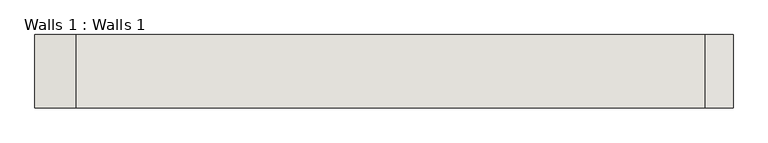
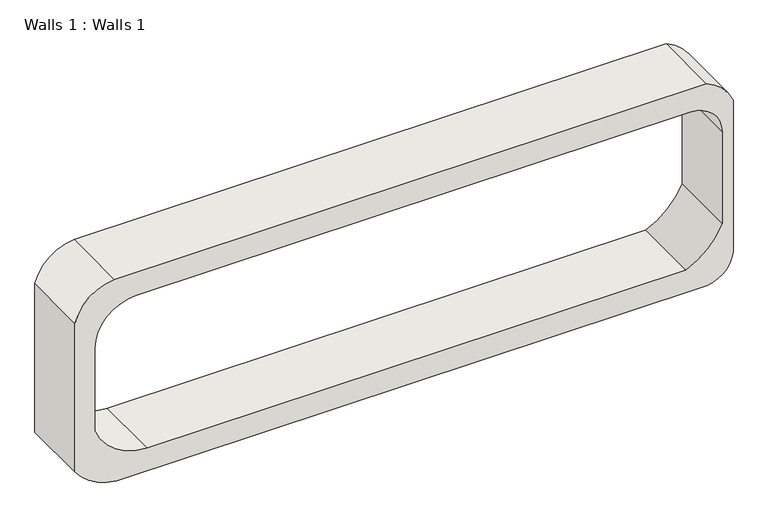
"""IFC4 building model written with IfcOpenShell, lengths in millimetres: wall geometry, Walls 1 : Walls 1."""

from ifc_helpers import new_model, si_unit, point, frame, frame_2d, origin, place, context, project, spatial, polyline, circle_curve, trimmed, segment, composite_curve, outline, extrude, source, transform, mapped, element, save


def walls_1_walls_1_13ff75f0(model_context):
    return source(origin(), model_context, "Body", "SweptSolid", [
        extrude(outline(composite_curve([segment(polyline([(6096.0, 5427.1580605), (6096.0, -4067.3110345)]), True, "CONTINUOUS"), segment(trimmed(circle_curve(frame_2d((5400.2481258, -4018.635718)), 697.4524764), [point((6096.0, -4067.3110345))], [point((5569.0, -4695.3651778))], False, "CARTESIAN"), True, "CONTINUOUS"), segment(polyline([(5569.0, -4695.3651778), (3048.0, -4695.3651778)]), True, "CONTINUOUS"), segment(trimmed(circle_curve(frame_2d((3589.3605138, -3935.5372859)), 932.9574649), [point((3048.0, -4695.3651778))], [point((2660.65, -4024.4552975))], False, "CARTESIAN"), True, "CONTINUOUS"), segment(polyline([(2660.65, -4024.4552975), (2660.65, 5350.9580605)]), True, "CONTINUOUS"), segment(trimmed(circle_curve(frame_2d((3133.5370241, 5386.466107)), 474.2182609), [point((2660.65, 5350.9580605))], [point((3086.3896536, 5858.3348222))], False, "CARTESIAN"), True, "CONTINUOUS"), segment(polyline([(3086.3896536, 5858.3348222), (5664.8232384, 5858.3348222)]), True, "CONTINUOUS"), segment(trimmed(circle_curve(frame_2d((5359.8751992, 5122.2100213)), 796.7891998), [point((5664.8232384, 5858.3348222))], [point((6096.0, 5427.1580605))], False, "CARTESIAN"), True, "CONTINUOUS")], self_intersect=False), holes=[composite_curve([segment(trimmed(circle_curve(frame_2d((5188.0, 5173.1580605)), 508.0), [point((5696.0, 5173.1580605))], [point((5188.0, 5681.1580605))], True, "CARTESIAN"), True, "CONTINUOUS"), segment(polyline([(5188.0, 5681.1580605), (3632.2, 5681.1580605)]), True, "CONTINUOUS"), segment(trimmed(circle_curve(frame_2d((4082.0319719, 4647.1260886)), 1127.6395354), [point((3632.2, 5681.1580605))], [point((3048.0, 5096.9580605))], True, "CARTESIAN"), True, "CONTINUOUS"), segment(polyline([(3048.0, 5096.9580605), (3048.0, -3534.849777)]), True, "CONTINUOUS"), segment(trimmed(circle_curve(frame_2d((3956.0772883, -3520.6998691)), 908.1875255), [point((3048.0, -3534.849777))], [point((3632.2, -4369.1738425))], True, "CARTESIAN"), True, "CONTINUOUS"), segment(polyline([(3632.2, -4369.1738425), (5035.6, -4369.1738425)]), True, "CONTINUOUS"), segment(trimmed(circle_curve(frame_2d((5035.6, -3708.7738425)), 660.4), [point((5035.6, -4369.1738425))], [point((5696.0, -3708.7738425))], True, "CARTESIAN"), True, "CONTINUOUS"), segment(polyline([(5696.0, -3708.7738425), (5696.0, 5173.1580605)]), True, "CONTINUOUS")], self_intersect=False)]), frame((0.0, -4049.3114058, 0.0), z_axis=(0.0, 1.0, 0.0), x_axis=(0.0, 0.0, 1.0)), (0.0, 0.0, 1.0), 1110.5603133),
    ])


if __name__ == "__main__":
    model = new_model("IFC4")
    model_context = context("Model", 3, world=origin())
    ifc_project = project(units=[si_unit("LENGTHUNIT", "METRE", prefix="MILLI")], contexts=[model_context])
    site = spatial("IfcSite", under=ifc_project)
    building = spatial("IfcBuilding", under=site)
    placement = place(None, origin())
    walls_1_walls_1_shape = walls_1_walls_1_13ff75f0(model_context)
    element("IfcWall", 1, ObjectType="Walls 1 : Walls 1", at=placement, inside=building, context=model_context, shape_type="MappedRepresentation", body=[
        mapped(walls_1_walls_1_shape, transform((0.0, 0.0, 0.0), x_axis=(1.0, 0.0, 0.0), y_axis=(0.0, 1.0, 0.0), z_axis=(0.0, 0.0, 1.0))),
    ])
    save(model, "model.ifc")

# Revit data of these elements
# Element 1 (IfcWall, "Walls 1 : Walls 1")
#   Materials on its faces: "Default Wall"
# Materials
#   "Default Wall": colour RGB 80 80 80, transparency 0
